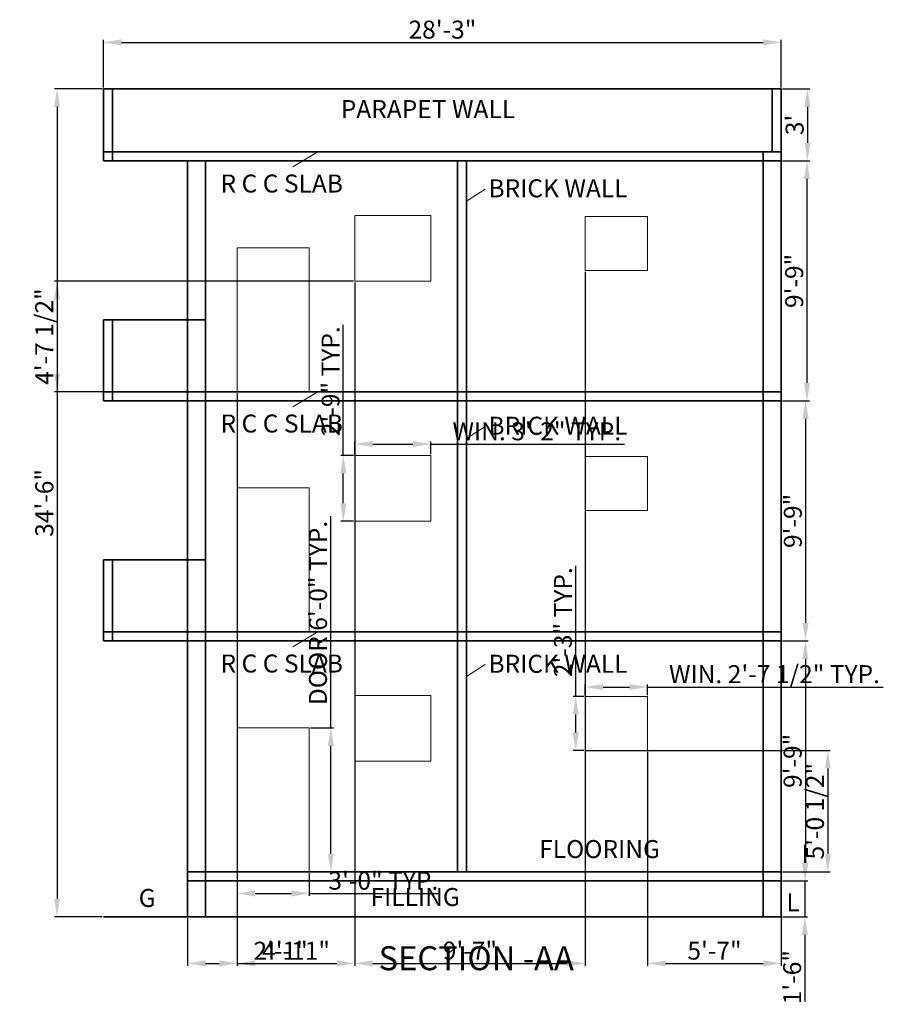
# Model space of a CAD drawing. Units: inches. Extents: x 2044 to 3644, y 808 to 1988.
# Tile 4 of 4: x 2762 to 3194, y 1496 to 1988. Entities that reach past the tile are written whole.
import ezdxf

# ---------------------------------------------------------------- set-up
doc = ezdxf.new("R2010")
doc.units = ezdxf.units.IN
for name, color, linetype, lineweight in [('A-ANNO-DIMS', 2, 'Continuous', 18), ('A-ANNO-SYMB', 2, 'Continuous', 18), ('A-ANNO-TEXT', 7, 'Continuous', 18), ('A-ANNO-TITL', 7, 'Continuous', 25), ('A-DOOR', 4, 'Continuous', 18), ('A-GLAZ', 4, 'Continuous', 18), ('A-SECT', 7, 'Continuous', 35)]:
    doc.layers.add(name, color=color, linetype=linetype, lineweight=lineweight)
doc.styles.get("Standard").update_dxf_attribs({"font": 'arial.ttf'})
doc.dimstyles.new('ISO-25', dxfattribs={"dimtxt": 9, "dimasz": 9, "dimexe": 1.25, "dimexo": 0.625, "dimtad": 1, "dimdec": 1, "dimrnd": 9, "dimlunit": 3, "dimtxsty": 'Standard', "dimcen": 2.5, "dimadec": 0, "dimazin": 0, "dimtfac": 1, "dimtdec": 1, "dimtmove": 0, "dimatfit": 3, "dimfxl": 1, "dimarcsym": 0})

# ---------------------------------------------------------------- blocks, each defined once
blk = doc.blocks.new('*D12')
at = {"layer": 'A-ANNO-DIMS', "color": 0, "lineweight": -2, "transparency": 16777216}
for p, q in [((3143.61, 1953.83), (3157.28, 1953.83)), ((3156.03, 1944.83), (3156.03, 1926.83)), ((3143.61, 1917.83), (3157.28, 1917.83))]:
    blk.add_line(p, q, dxfattribs=at)
at = {"layer": 'A-ANNO-DIMS', "color": 0, "transparency": 16777216}
for points in [[(3154.53, 1944.83), (3157.53, 1944.83), (3156.03, 1953.83)], [(3154.53, 1926.83), (3157.53, 1926.83), (3156.03, 1917.83)]]:
    blk.add_solid(points, dxfattribs=at)
at = {"layer": 'Defpoints', "color": 0, "transparency": 16777216}
for p in [(3142.98, 1953.83), (3142.98, 1917.83), (3156.03, 1917.83)]:
    blk.add_point(p, dxfattribs=at)
at = {"layer": 'A-ANNO-DIMS', "color": 0, "transparency": 16777216, "insert": (3150.81, 1935.83), "char_height": 9, "attachment_point": 5, "rotation": 90}
blk.add_mtext("3'", dxfattribs=at)
blk = doc.blocks.new('*D13')
at = {"layer": 'A-ANNO-DIMS', "color": 0, "lineweight": -2, "transparency": 16777216}
for p, q in [((3143.61, 1917.83), (3157.05, 1917.83)), ((3155.8, 1908.83), (3155.8, 1806.83)), ((3143.61, 1797.83), (3157.05, 1797.83))]:
    blk.add_line(p, q, dxfattribs=at)
at = {"layer": 'A-ANNO-DIMS', "color": 0, "transparency": 16777216}
for points in [[(3154.3, 1908.83), (3157.3, 1908.83), (3155.8, 1917.83)], [(3154.3, 1806.83), (3157.3, 1806.83), (3155.8, 1797.83)]]:
    blk.add_solid(points, dxfattribs=at)
at = {"layer": 'Defpoints', "color": 0, "transparency": 16777216}
for p in [(3142.98, 1917.83), (3142.98, 1797.83), (3155.8, 1797.83)]:
    blk.add_point(p, dxfattribs=at)
at = {"layer": 'A-ANNO-DIMS', "color": 0, "transparency": 16777216, "insert": (3150.58, 1857.83), "char_height": 9, "attachment_point": 5, "rotation": 90}
blk.add_mtext('9\'-9"', dxfattribs=at)
blk = doc.blocks.new('*D14')
at = {"layer": 'A-ANNO-DIMS', "color": 0, "lineweight": -2, "transparency": 16777216}
for p, q in [((3143.61, 1797.83), (3156.36, 1797.83)), ((3155.11, 1788.83), (3155.11, 1686.83)), ((3143.61, 1677.83), (3156.36, 1677.83))]:
    blk.add_line(p, q, dxfattribs=at)
at = {"layer": 'A-ANNO-DIMS', "color": 0, "transparency": 16777216}
for points in [[(3153.61, 1788.83), (3156.61, 1788.83), (3155.11, 1797.83)], [(3153.61, 1686.83), (3156.61, 1686.83), (3155.11, 1677.83)]]:
    blk.add_solid(points, dxfattribs=at)
at = {"layer": 'Defpoints', "color": 0, "transparency": 16777216}
for p in [(3142.98, 1797.83), (3142.98, 1677.83), (3155.11, 1677.83)]:
    blk.add_point(p, dxfattribs=at)
at = {"layer": 'A-ANNO-DIMS', "color": 0, "transparency": 16777216, "insert": (3149.89, 1737.83), "char_height": 9, "attachment_point": 5, "rotation": 90}
blk.add_mtext('9\'-9"', dxfattribs=at)
blk = doc.blocks.new('*D15')
at = {"layer": 'A-ANNO-DIMS', "color": 0, "lineweight": -2, "transparency": 16777216}
for p, q in [((3143.61, 1677.83), (3156.27, 1677.83)), ((3155.02, 1668.83), (3155.02, 1566.83)), ((3143.61, 1557.83), (3156.27, 1557.83))]:
    blk.add_line(p, q, dxfattribs=at)
at = {"layer": 'A-ANNO-DIMS', "color": 0, "transparency": 16777216}
for points in [[(3153.52, 1668.83), (3156.52, 1668.83), (3155.02, 1677.83)], [(3153.52, 1566.83), (3156.52, 1566.83), (3155.02, 1557.83)]]:
    blk.add_solid(points, dxfattribs=at)
at = {"layer": 'Defpoints', "color": 0, "transparency": 16777216}
for p in [(3142.98, 1677.83), (3142.98, 1557.83), (3155.02, 1557.83)]:
    blk.add_point(p, dxfattribs=at)
at = {"layer": 'A-ANNO-DIMS', "color": 0, "transparency": 16777216, "insert": (3149.8, 1617.83), "char_height": 9, "attachment_point": 5, "rotation": 90}
blk.add_mtext('9\'-9"', dxfattribs=at)
blk = doc.blocks.new('*D16')
at = {"layer": 'A-ANNO-DIMS', "color": 0, "lineweight": -2, "transparency": 16777216}
for p, q in [((3154.79, 1566.83), (3154.79, 1575.83)), ((3143.61, 1557.83), (3156.04, 1557.83)), ((3154.79, 1557.83), (3154.79, 1539.83)), ((3143.61, 1539.83), (3156.04, 1539.83)), ((3154.79, 1530.83), (3154.79, 1497.51))]:
    blk.add_line(p, q, dxfattribs=at)
at = {"layer": 'A-ANNO-DIMS', "color": 0, "transparency": 16777216}
for points in [[(3153.29, 1566.83), (3156.29, 1566.83), (3154.79, 1557.83)], [(3153.29, 1530.83), (3156.29, 1530.83), (3154.79, 1539.83)]]:
    blk.add_solid(points, dxfattribs=at)
at = {"layer": 'Defpoints', "color": 0, "transparency": 16777216}
for p in [(3142.98, 1557.83), (3142.98, 1539.83), (3154.79, 1539.83)]:
    blk.add_point(p, dxfattribs=at)
at = {"layer": 'A-ANNO-DIMS', "color": 0, "transparency": 16777216, "insert": (3149.57, 1509.67), "char_height": 9, "attachment_point": 5, "rotation": 90}
blk.add_mtext('1\'-6"', dxfattribs=at)
blk = doc.blocks.new('DOOR-36-SECTION')
for p, q in [((0, 0), (0, 72)), ((0, 72), (36, 72)), ((36, 72), (36, 0))]:
    blk.add_line(p, q)
blk = doc.blocks.new('WIN-WIDE-SECTION')
blk.add_lwpolyline([(0, 32.89), (38.09, 32.89), (38.09, 0), (0, 0)], close=True)
blk = doc.blocks.new('WIN-NARROW-SECTION')
blk.add_lwpolyline([(0, 27.02), (31.27, 27.02), (31.27, 0), (0, 0)], close=True)
blk = doc.blocks.new('*D45')
at = {"layer": 'A-ANNO-DIMS', "color": 0, "lineweight": -2, "transparency": 16777216}
for p, q in [((2917.67, 1634.33), (2917.67, 1740.21)), ((2907.49, 1634.33), (2918.92, 1634.33)), ((2917.67, 1571.33), (2917.67, 1625.33)), ((2907.49, 1562.33), (2918.92, 1562.33))]:
    blk.add_line(p, q, dxfattribs=at)
at = {"layer": 'A-ANNO-DIMS', "color": 0, "transparency": 16777216}
for points in [[(2916.17, 1625.33), (2919.17, 1625.33), (2917.67, 1634.33)], [(2916.17, 1571.33), (2919.17, 1571.33), (2917.67, 1562.33)]]:
    blk.add_solid(points, dxfattribs=at)
at = {"layer": 'Defpoints', "color": 0, "transparency": 16777216}
for p in [(2906.87, 1634.33), (2917.67, 1634.33), (2906.87, 1562.33)]:
    blk.add_point(p, dxfattribs=at)
at = {"layer": 'A-ANNO-DIMS', "color": 0, "transparency": 16777216, "insert": (2912.38, 1691.77), "char_height": 9, "attachment_point": 5, "rotation": 90}
blk.add_mtext('DOOR 6\'-0" TYP.', dxfattribs=at)
blk = doc.blocks.new('*D46')
at = {"layer": 'A-ANNO-DIMS', "color": 0, "lineweight": -2, "transparency": 16777216}
for p, q in [((2870.87, 1561.71), (2870.87, 1550.28)), ((2906.87, 1561.71), (2906.87, 1550.28)), ((2879.87, 1551.53), (2897.87, 1551.53)), ((2906.87, 1551.53), (2971.97, 1551.53))]:
    blk.add_line(p, q, dxfattribs=at)
at = {"layer": 'A-ANNO-DIMS', "color": 0, "transparency": 16777216}
for points in [[(2879.87, 1553.03), (2879.87, 1550.03), (2870.87, 1551.53)], [(2897.87, 1553.03), (2897.87, 1550.03), (2906.87, 1551.53)]]:
    blk.add_solid(points, dxfattribs=at)
at = {"layer": 'Defpoints', "color": 0, "transparency": 16777216}
for p in [(2870.87, 1562.33), (2906.87, 1562.33), (2906.87, 1551.53)]:
    blk.add_point(p, dxfattribs=at)
at = {"layer": 'A-ANNO-DIMS', "color": 0, "transparency": 16777216, "insert": (2943.92, 1556.76), "char_height": 9, "attachment_point": 5}
blk.add_mtext('3\'-0" TYP.', dxfattribs=at)
blk = doc.blocks.new('*D47')
at = {"layer": 'A-ANNO-DIMS', "color": 0, "lineweight": -2, "transparency": 16777216}
for p, q in [((2929.63, 1771.17), (2929.63, 1777.5)), ((2967.71, 1771.17), (2967.71, 1777.5)), ((2938.63, 1776.25), (2958.71, 1776.25)), ((2967.71, 1776.25), (3064.62, 1776.25))]:
    blk.add_line(p, q, dxfattribs=at)
at = {"layer": 'A-ANNO-DIMS', "color": 0, "transparency": 16777216}
for points in [[(2938.63, 1777.75), (2938.63, 1774.75), (2929.63, 1776.25)], [(2958.71, 1777.75), (2958.71, 1774.75), (2967.71, 1776.25)]]:
    blk.add_solid(points, dxfattribs=at)
at = {"layer": 'Defpoints', "color": 0, "transparency": 16777216}
for p in [(2967.71, 1776.25), (2929.63, 1770.54), (2967.71, 1770.54)]:
    blk.add_point(p, dxfattribs=at)
at = {"layer": 'A-ANNO-DIMS', "color": 0, "transparency": 16777216, "insert": (3020.67, 1781.48), "char_height": 9, "attachment_point": 5}
blk.add_mtext('WIN. 3\'-2" TYP.', dxfattribs=at)
blk = doc.blocks.new('*D48')
at = {"layer": 'A-ANNO-DIMS', "color": 0, "lineweight": -2, "transparency": 16777216}
for p, q in [((2923.91, 1770.54), (2923.91, 1835.8)), ((2929, 1770.54), (2922.66, 1770.54)), ((2923.91, 1746.65), (2923.91, 1761.54)), ((2929, 1737.65), (2922.66, 1737.65))]:
    blk.add_line(p, q, dxfattribs=at)
at = {"layer": 'A-ANNO-DIMS', "color": 0, "transparency": 16777216}
for points in [[(2922.41, 1761.54), (2925.41, 1761.54), (2923.91, 1770.54)], [(2922.41, 1746.65), (2925.41, 1746.65), (2923.91, 1737.65)]]:
    blk.add_solid(points, dxfattribs=at)
at = {"layer": 'Defpoints', "color": 0, "transparency": 16777216}
for p in [(2923.91, 1770.54), (2929.63, 1770.54), (2929.63, 1737.65)]:
    blk.add_point(p, dxfattribs=at)
at = {"layer": 'A-ANNO-DIMS', "color": 0, "transparency": 16777216, "insert": (2918.69, 1807.67), "char_height": 9, "attachment_point": 5, "rotation": 90}
blk.add_mtext('2\'-9" TYP.', dxfattribs=at)
blk = doc.blocks.new('*D49')
at = {"layer": 'A-ANNO-DIMS', "color": 0, "lineweight": -2, "transparency": 16777216}
for p, q in [((3044.85, 1650.69), (3044.85, 1656)), ((3053.85, 1654.75), (3067.12, 1654.75)), ((3076.12, 1650.69), (3076.12, 1656)), ((3076.12, 1654.75), (3193.99, 1654.75))]:
    blk.add_line(p, q, dxfattribs=at)
at = {"layer": 'A-ANNO-DIMS', "color": 0, "transparency": 16777216}
for points in [[(3053.85, 1656.25), (3053.85, 1653.25), (3044.85, 1654.75)], [(3067.12, 1656.25), (3067.12, 1653.25), (3076.12, 1654.75)]]:
    blk.add_solid(points, dxfattribs=at)
at = {"layer": 'Defpoints', "color": 0, "transparency": 16777216}
for p in [(3076.12, 1654.75), (3044.85, 1650.06), (3076.12, 1650.06)]:
    blk.add_point(p, dxfattribs=at)
at = {"layer": 'A-ANNO-DIMS', "color": 0, "transparency": 16777216, "insert": (3139.55, 1660.03), "char_height": 9, "attachment_point": 5}
blk.add_mtext('WIN. 2\'-7 1/2" TYP.', dxfattribs=at)
blk = doc.blocks.new('*D50')
at = {"layer": 'A-ANNO-DIMS', "color": 0, "lineweight": -2, "transparency": 16777216}
for p, q in [((3040.16, 1650.06), (3040.16, 1715.32)), ((3044.22, 1650.06), (3038.91, 1650.06)), ((3040.16, 1632.05), (3040.16, 1641.06)), ((3044.22, 1623.05), (3038.91, 1623.05))]:
    blk.add_line(p, q, dxfattribs=at)
at = {"layer": 'A-ANNO-DIMS', "color": 0, "transparency": 16777216}
for points in [[(3038.66, 1641.06), (3041.66, 1641.06), (3040.16, 1650.06)], [(3038.66, 1632.05), (3041.66, 1632.05), (3040.16, 1623.05)]]:
    blk.add_solid(points, dxfattribs=at)
at = {"layer": 'Defpoints', "color": 0, "transparency": 16777216}
for p in [(3040.16, 1650.06), (3044.85, 1650.06), (3044.85, 1623.05)]:
    blk.add_point(p, dxfattribs=at)
at = {"layer": 'A-ANNO-DIMS', "color": 0, "transparency": 16777216, "insert": (3034.93, 1687.19), "char_height": 9, "attachment_point": 5, "rotation": 90}
blk.add_mtext('2\'-3" TYP.', dxfattribs=at)
blk = doc.blocks.new('*D68')
at = {"layer": 'A-ANNO-DIMS', "color": 0, "lineweight": -2, "transparency": 16777216}
for p, q in [((2803.98, 1954.46), (2803.98, 1978.33)), ((2812.98, 1977.08), (3133.98, 1977.08)), ((3142.98, 1954.46), (3142.98, 1978.33))]:
    blk.add_line(p, q, dxfattribs=at)
at = {"layer": 'A-ANNO-DIMS', "color": 0, "transparency": 16777216}
for points in [[(2812.98, 1978.58), (2812.98, 1975.58), (2803.98, 1977.08)], [(3133.98, 1978.58), (3133.98, 1975.58), (3142.98, 1977.08)]]:
    blk.add_solid(points, dxfattribs=at)
at = {"layer": 'Defpoints', "color": 0, "transparency": 16777216}
for p in [(3142.98, 1977.08), (2803.98, 1953.83), (3142.98, 1953.83)]:
    blk.add_point(p, dxfattribs=at)
at = {"layer": 'A-ANNO-DIMS', "color": 0, "transparency": 16777216, "insert": (2973.48, 1982.31), "char_height": 9, "attachment_point": 5}
blk.add_mtext('28\'-3"', dxfattribs=at)
blk = doc.blocks.new('*D69')
at = {"layer": 'A-ANNO-DIMS', "color": 0, "lineweight": -2, "transparency": 16777216}
for p, q in [((2803.36, 1953.83), (2779.48, 1953.83)), ((2780.73, 1944.83), (2780.73, 1548.83)), ((2803.36, 1539.83), (2779.48, 1539.83))]:
    blk.add_line(p, q, dxfattribs=at)
at = {"layer": 'A-ANNO-DIMS', "color": 0, "transparency": 16777216}
for points in [[(2779.23, 1944.83), (2782.23, 1944.83), (2780.73, 1953.83)], [(2779.23, 1548.83), (2782.23, 1548.83), (2780.73, 1539.83)]]:
    blk.add_solid(points, dxfattribs=at)
at = {"layer": 'Defpoints', "color": 0, "transparency": 16777216}
for p in [(2803.98, 1953.83), (2780.73, 1539.83), (2803.98, 1539.83)]:
    blk.add_point(p, dxfattribs=at)
at = {"layer": 'A-ANNO-DIMS', "color": 0, "transparency": 16777216, "insert": (2775.51, 1746.83), "char_height": 9, "attachment_point": 5, "rotation": 90}
blk.add_mtext('34\'-6"', dxfattribs=at)
blk = doc.blocks.new('*D70')
at = {"layer": 'A-ANNO-DIMS', "color": 0, "lineweight": -2, "transparency": 16777216}
for p, q in [((2870.87, 1561.71), (2870.87, 1515.33)), ((2845.98, 1539.21), (2845.98, 1515.33)), ((2854.98, 1516.58), (2861.87, 1516.58)), ((2870.87, 1516.58), (2905.19, 1516.58))]:
    blk.add_line(p, q, dxfattribs=at)
at = {"layer": 'A-ANNO-DIMS', "color": 0, "transparency": 16777216}
for points in [[(2854.98, 1518.08), (2854.98, 1515.08), (2845.98, 1516.58)], [(2861.87, 1518.08), (2861.87, 1515.08), (2870.87, 1516.58)]]:
    blk.add_solid(points, dxfattribs=at)
at = {"layer": 'Defpoints', "color": 0, "transparency": 16777216}
for p in [(2870.87, 1562.33), (2845.98, 1539.83), (2870.87, 1516.58)]:
    blk.add_point(p, dxfattribs=at)
at = {"layer": 'A-ANNO-DIMS', "color": 0, "transparency": 16777216, "insert": (2892.53, 1521.73), "char_height": 9, "attachment_point": 5}
blk.add_mtext('2\'-1"', dxfattribs=at)
blk = doc.blocks.new('*D71')
at = {"layer": 'A-ANNO-DIMS', "color": 0, "lineweight": -2, "transparency": 16777216}
for p, q in [((2929.63, 1857.03), (2929.63, 1515.33)), ((2870.87, 1801.71), (2870.87, 1515.33)), ((2879.87, 1516.58), (2920.63, 1516.58))]:
    blk.add_line(p, q, dxfattribs=at)
at = {"layer": 'A-ANNO-DIMS', "color": 0, "transparency": 16777216}
for points in [[(2879.87, 1518.08), (2879.87, 1515.08), (2870.87, 1516.58)], [(2920.63, 1518.08), (2920.63, 1515.08), (2929.63, 1516.58)]]:
    blk.add_solid(points, dxfattribs=at)
at = {"layer": 'Defpoints', "color": 0, "transparency": 16777216}
for p in [(2929.63, 1857.65), (2870.87, 1802.33), (2929.63, 1516.58)]:
    blk.add_point(p, dxfattribs=at)
at = {"layer": 'A-ANNO-DIMS', "color": 0, "transparency": 16777216, "insert": (2900.25, 1521.73), "char_height": 9, "attachment_point": 5}
blk.add_mtext('4\'-11"', dxfattribs=at)
blk = doc.blocks.new('*D72')
at = {"layer": 'A-ANNO-DIMS', "color": 0, "lineweight": -2, "transparency": 16777216}
for p, q in [((3044.85, 1862.42), (3044.85, 1515.33)), ((2929.63, 1857.03), (2929.63, 1515.33)), ((2938.63, 1516.58), (3035.85, 1516.58))]:
    blk.add_line(p, q, dxfattribs=at)
at = {"layer": 'A-ANNO-DIMS', "color": 0, "transparency": 16777216}
for points in [[(2938.63, 1518.08), (2938.63, 1515.08), (2929.63, 1516.58)], [(3035.85, 1518.08), (3035.85, 1515.08), (3044.85, 1516.58)]]:
    blk.add_solid(points, dxfattribs=at)
at = {"layer": 'Defpoints', "color": 0, "transparency": 16777216}
for p in [(3044.85, 1863.05), (2929.63, 1857.65), (3044.85, 1516.58)]:
    blk.add_point(p, dxfattribs=at)
at = {"layer": 'A-ANNO-DIMS', "color": 0, "transparency": 16777216, "insert": (2987.24, 1521.8), "char_height": 9, "attachment_point": 5}
blk.add_mtext('9\'-7"', dxfattribs=at)
blk = doc.blocks.new('*D73')
at = {"layer": 'A-ANNO-DIMS', "color": 0, "lineweight": -2, "transparency": 16777216}
for p, q in [((2929, 1857.65), (2779.48, 1857.65)), ((2780.73, 1848.65), (2780.73, 1811.33)), ((2870.24, 1802.33), (2779.48, 1802.33))]:
    blk.add_line(p, q, dxfattribs=at)
at = {"layer": 'A-ANNO-DIMS', "color": 0, "transparency": 16777216}
for points in [[(2779.23, 1848.65), (2782.23, 1848.65), (2780.73, 1857.65)], [(2779.23, 1811.33), (2782.23, 1811.33), (2780.73, 1802.33)]]:
    blk.add_solid(points, dxfattribs=at)
at = {"layer": 'Defpoints', "color": 0, "transparency": 16777216}
for p in [(2929.63, 1857.65), (2780.73, 1802.33), (2870.87, 1802.33)]:
    blk.add_point(p, dxfattribs=at)
at = {"layer": 'A-ANNO-DIMS', "color": 0, "transparency": 16777216, "insert": (2775.45, 1829.99), "char_height": 9, "attachment_point": 5, "rotation": 90}
blk.add_mtext('4\'-7 1/2"', dxfattribs=at)
blk = doc.blocks.new('*D74')
at = {"layer": 'A-ANNO-DIMS', "color": 0, "lineweight": -2, "transparency": 16777216}
for p, q in [((3045.47, 1623.05), (3167.48, 1623.05)), ((3166.23, 1614.05), (3166.23, 1571.33)), ((3143.61, 1562.33), (3167.48, 1562.33))]:
    blk.add_line(p, q, dxfattribs=at)
at = {"layer": 'A-ANNO-DIMS', "color": 0, "transparency": 16777216}
for points in [[(3164.73, 1614.05), (3167.73, 1614.05), (3166.23, 1623.05)], [(3164.73, 1571.33), (3167.73, 1571.33), (3166.23, 1562.33)]]:
    blk.add_solid(points, dxfattribs=at)
at = {"layer": 'Defpoints', "color": 0, "transparency": 16777216}
for p in [(3044.85, 1623.05), (3142.98, 1562.33), (3166.23, 1562.33)]:
    blk.add_point(p, dxfattribs=at)
at = {"layer": 'A-ANNO-DIMS', "color": 0, "transparency": 16777216, "insert": (3160.95, 1592.69), "char_height": 9, "attachment_point": 5, "rotation": 90}
blk.add_mtext('5\'-0 1/2"', dxfattribs=at)
blk = doc.blocks.new('*D75')
at = {"layer": 'A-ANNO-DIMS', "color": 0, "lineweight": -2, "transparency": 16777216}
for p, q in [((3076.12, 1622.42), (3076.12, 1515.33)), ((3142.98, 1561.71), (3142.98, 1515.33)), ((3085.12, 1516.58), (3133.98, 1516.58))]:
    blk.add_line(p, q, dxfattribs=at)
at = {"layer": 'A-ANNO-DIMS', "color": 0, "transparency": 16777216}
for points in [[(3085.12, 1518.08), (3085.12, 1515.08), (3076.12, 1516.58)], [(3133.98, 1518.08), (3133.98, 1515.08), (3142.98, 1516.58)]]:
    blk.add_solid(points, dxfattribs=at)
at = {"layer": 'Defpoints', "color": 0, "transparency": 16777216}
for p in [(3076.12, 1623.05), (3142.98, 1562.33), (3142.98, 1516.58)]:
    blk.add_point(p, dxfattribs=at)
at = {"layer": 'A-ANNO-DIMS', "color": 0, "transparency": 16777216, "insert": (3109.55, 1521.79), "char_height": 9, "attachment_point": 5}
blk.add_mtext('5\'-7"', dxfattribs=at)

msp = doc.modelspace()

# ---------------------------------------------------------------- linework, layer by layer
at = {"layer": 'A-ANNO-TEXT'}
for p, q in [((2911.15, 1922.33), (2898.71, 1914.91)), ((2985.48, 1897.77), (2994.81, 1903.71)), ((2911.15, 1802.33), (2898.71, 1794.91)), ((2985.48, 1779.05), (2994.81, 1785)), ((2911.15, 1682.33), (2898.71, 1674.91)), ((2985.48, 1660.02), (2994.81, 1665.97))]:
    msp.add_line(p, q, dxfattribs=at)
at = {"layer": 'A-SECT'}
for p, q in [((2803.98, 1953.83), (3142.98, 1953.83)), ((2803.98, 1917.83), (2803.98, 1953.83)), ((2808.48, 1917.83), (2808.48, 1953.83)), ((3138.48, 1953.83), (3138.48, 1922.33)), ((3142.98, 1953.83), (3142.98, 1922.33)), ((2803.98, 1922.33), (3142.98, 1922.33)), ((3133.98, 1539.83), (3133.98, 1922.33)), ((3142.98, 1539.83), (3142.98, 1922.33)), ((2803.98, 1917.83), (3142.98, 1917.83)), ((2845.98, 1539.83), (2845.98, 1917.83)), ((2854.98, 1539.83), (2854.98, 1917.83)), ((2980.98, 1562.33), (2980.98, 1917.83)), ((2985.48, 1562.33), (2985.48, 1917.83)), ((2803.98, 1838.33), (2854.98, 1838.33)), ((2803.98, 1797.83), (2803.98, 1838.33)), ((2808.48, 1797.83), (2808.48, 1838.33)), ((2803.98, 1802.33), (3142.98, 1802.33)), ((2803.98, 1797.83), (3142.98, 1797.83)), ((2803.98, 1718.33), (2854.98, 1718.33)), ((2803.98, 1677.83), (2803.98, 1718.33)), ((2808.48, 1677.83), (2808.48, 1718.33)), ((2803.98, 1682.33), (3142.98, 1682.33)), ((2803.98, 1677.83), (3142.98, 1677.83)), ((2845.98, 1562.33), (3142.98, 1562.33)), ((2845.98, 1557.83), (3142.98, 1557.83)), ((2803.98, 1539.83), (3142.98, 1539.83))]:
    msp.add_line(p, q, dxfattribs=at)

# ---------------------------------------------------------------- block references
at = {"layer": 'A-DOOR'}
for p in [(2870.87, 1802.33), (2870.87, 1682.33), (2870.87, 1562.33)]:
    msp.add_blockref('DOOR-36-SECTION', p, dxfattribs=at)
at = {"layer": 'A-GLAZ'}
for name, p in [('WIN-WIDE-SECTION', (2929.63, 1857.65)), ('WIN-NARROW-SECTION', (3044.85, 1863.05)), ('WIN-WIDE-SECTION', (2929.63, 1737.65)), ('WIN-NARROW-SECTION', (3044.85, 1743.05)), ('WIN-WIDE-SECTION', (2929.63, 1617.65)), ('WIN-NARROW-SECTION', (3044.85, 1623.05))]:
    msp.add_blockref(name, p, dxfattribs=at)

# ---------------------------------------------------------------- texts
at = {"layer": 'A-ANNO-SYMB', "char_height": 9, "attachment_point": 1}
for s, insert in [('G', (2821.56, 1553.79)), ('L', (3145.52, 1551.67))]:
    msp.add_mtext_dynamic_manual_height_columns(s, width=19.1778, gutter_width=12.5, heights=[0], dxfattribs=dict(at, insert=insert))
at = {"layer": 'A-ANNO-TEXT', "char_height": 9, "attachment_point": 1}
for s, insert in [('PARAPET WALL', (2922.64, 1948.23)), ('R C C SLAB', (2862.48, 1911.02)), ('BRICK WALL', (2996.5, 1908.62)), ('R C C SLAB', (2862.48, 1791.02)), ('BRICK WALL', (2996.5, 1789.91)), ('R C C SLAB', (2862.48, 1671.02)), ('BRICK WALL', (2996.5, 1670.88)), ('FLOORING', (3021.87, 1578.23)), ('FILLING', (2937.51, 1554.26))]:
    msp.add_mtext_dynamic_manual_height_columns(s, width=134.103, gutter_width=12.5, heights=[0], dxfattribs=dict(at, insert=insert))
at = {"layer": 'A-ANNO-TITL', "insert": (2941.53, 1525.16), "char_height": 12, "attachment_point": 1}
msp.add_mtext_dynamic_manual_height_columns('SECTION -AA', width=134.103, gutter_width=12.5, heights=[0], dxfattribs=at)

# ---------------------------------------------------------------- dimensions: what is measured, and where the dimension line sits
at = {"layer": 'A-ANNO-DIMS'}
for base, p1, p2, picture, middle in [((3142.98, 1977.08), (2803.98, 1953.83), (3142.98, 1953.83), '*D68', (2973.48, 1982.31)), ((3044.85, 1516.58), (2929.63, 1857.65), (3044.85, 1863.05), '*D72', (2987.24, 1521.8)), ((2929.63, 1516.58), (2870.87, 1802.33), (2929.63, 1857.65), '*D71', (2900.25, 1521.73)), ((3142.98, 1516.58), (3076.12, 1623.05), (3142.98, 1562.33), '*D75', (3109.55, 1521.79)), ((2870.87, 1516.58), (2845.98, 1539.83), (2870.87, 1562.33), '*D70', (2892.53, 1521.73))]:
    dim = msp.add_linear_dim(base=base, p1=p1, p2=p2, dimstyle='ISO-25', override={"dimdec": 1, "dimlfac": 1, "dimrnd": 0, "dimzin": 1, "dimdsep": 46, "dimlunit": 4, "dimfrac": 2}, dxfattribs=at)
    dim.commit()
    dim.dimension.update_dxf_attribs({"geometry": picture, "text_midpoint": middle})
for base, p1, p2, override, picture, middle in [((2780.73, 1539.83), (2803.98, 1953.83), (2803.98, 1539.83), {"dimdec": 1, "dimlfac": 1, "dimrnd": 0, "dimzin": 1, "dimdsep": 46, "dimlunit": 4, "dimfrac": 2}, '*D69', (2775.51, 1746.83)), ((3156.03, 1917.83), (3142.98, 1953.83), (3142.98, 1917.83), {"dimclrd": 0, "dimclre": 0, "dimclrt": 0}, '*D12', (3150.81, 1935.83)), ((3155.8, 1797.83), (3142.98, 1917.83), (3142.98, 1797.83), {"dimclrd": 0, "dimclre": 0, "dimclrt": 0}, '*D13', (3150.58, 1857.83)), ((2780.73, 1802.33), (2929.63, 1857.65), (2870.87, 1802.33), {"dimdec": 1, "dimlfac": 1, "dimrnd": 0, "dimzin": 1, "dimdsep": 46, "dimlunit": 4, "dimfrac": 2}, '*D73', (2775.45, 1829.99)), ((3155.11, 1677.83), (3142.98, 1797.83), (3142.98, 1677.83), {"dimclrd": 0, "dimclre": 0, "dimclrt": 0}, '*D14', (3149.89, 1737.83)), ((3155.02, 1557.83), (3142.98, 1677.83), (3142.98, 1557.83), {"dimclrd": 0, "dimclre": 0, "dimclrt": 0}, '*D15', (3149.8, 1617.83)), ((3166.23, 1562.33), (3044.85, 1623.05), (3142.98, 1562.33), {"dimdec": 1, "dimlfac": 1, "dimrnd": 0, "dimzin": 1, "dimdsep": 46, "dimlunit": 4, "dimfrac": 2}, '*D74', (3160.95, 1592.69)), ((3154.79, 1539.83), (3142.98, 1557.83), (3142.98, 1539.83), {"dimclrd": 0, "dimclre": 0, "dimclrt": 0}, '*D16', (3149.57, 1509.67))]:
    dim = msp.add_linear_dim(base=base, p1=p1, p2=p2, angle=90, dimstyle='ISO-25', override=override, dxfattribs=at)
    dim.commit()
    dim.dimension.update_dxf_attribs({"geometry": picture, "text_midpoint": middle})
for base, p1, p2, text, picture, middle in [((2923.91, 1770.54), (2929.63, 1737.65), (2929.63, 1770.54), '<> TYP.', '*D48', (2918.69, 1807.67)), ((2917.67, 1634.33), (2906.87, 1562.33), (2906.87, 1634.33), 'DOOR <> TYP.', '*D45', (2912.38, 1691.77)), ((3040.16, 1650.06), (3044.85, 1623.05), (3044.85, 1650.06), '<> TYP.', '*D50', (3034.93, 1687.19))]:
    dim = msp.add_linear_dim(base=base, p1=p1, p2=p2, angle=90, text=text, dimstyle='ISO-25', override={"dimdec": 1, "dimlfac": 1, "dimrnd": 0, "dimzin": 1, "dimdsep": 46, "dimlunit": 4, "dimfrac": 2}, dxfattribs=at)
    dim.commit()
    dim.dimension.update_dxf_attribs({"geometry": picture, "text_midpoint": middle})
for base, p1, p2, text, picture, middle in [((2967.71, 1776.25), (2929.63, 1770.54), (2967.71, 1770.54), 'WIN. <> TYP.', '*D47', (3020.67, 1781.48)), ((3076.12, 1654.75), (3044.85, 1650.06), (3076.12, 1650.06), 'WIN. <> TYP.', '*D49', (3139.55, 1660.03)), ((2906.87, 1551.53), (2870.87, 1562.33), (2906.87, 1562.33), '<> TYP.', '*D46', (2943.92, 1556.76))]:
    dim = msp.add_linear_dim(base=base, p1=p1, p2=p2, text=text, dimstyle='ISO-25', override={"dimdec": 1, "dimlfac": 1, "dimrnd": 0, "dimzin": 1, "dimdsep": 46, "dimlunit": 4, "dimfrac": 2}, dxfattribs=at)
    dim.commit()
    dim.dimension.update_dxf_attribs({"geometry": picture, "text_midpoint": middle})

doc.saveas('drawing.dxf')
